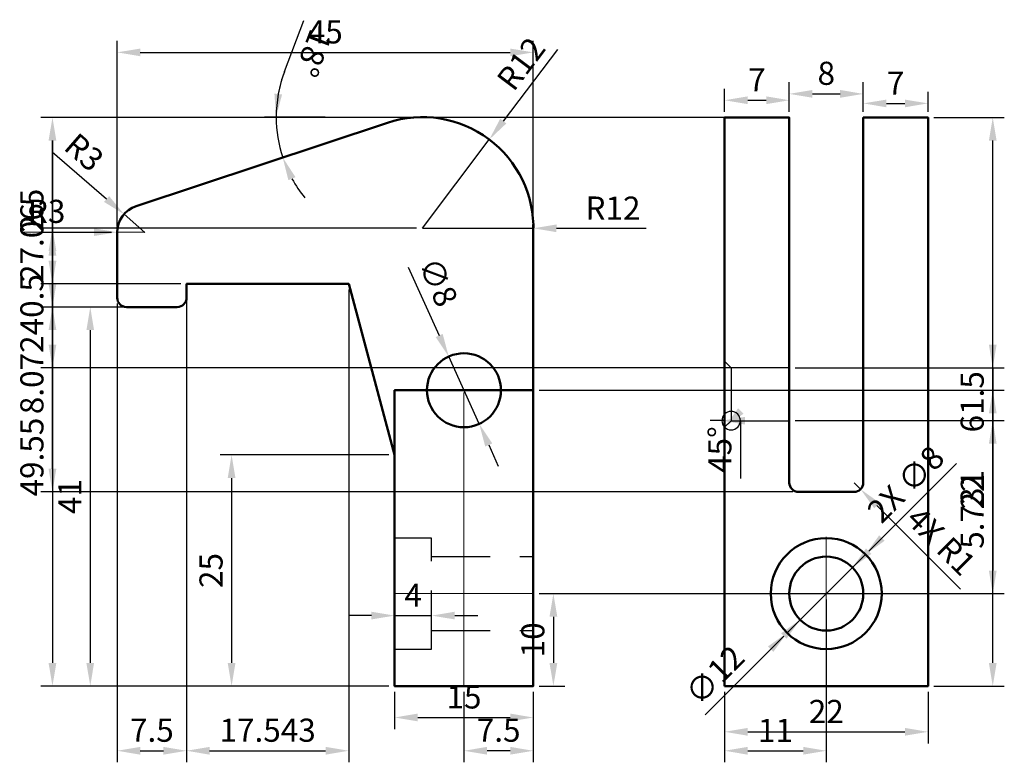
# Model space of a CAD drawing. Units: millimetres. Extents: x 28 to 135, y 8 to 88.
import ezdxf

# ---------------------------------------------------------------- set-up
doc = ezdxf.new("R2010")
doc.units = ezdxf.units.MM
doc.linetypes.add('CENTER', pattern=[50.8, 31.75, -6.35, 6.35, -6.35])
doc.linetypes.add('HIDDEN', pattern=[9.525, 6.35, -3.175])
for name, color, linetype, lineweight in [('M-CNTR', 4, 'CENTER', 18), ('M-CONS', 8, 'Continuous', 13), ('M-DIMS', 2, 'Continuous', 25), ('M-HIDN', 3, 'HIDDEN', 25), ('M-OUTL', 7, 'Continuous', 50)]:
    doc.layers.add(name, color=color, linetype=linetype, lineweight=lineweight)
doc.styles.get("Standard").update_dxf_attribs({"font": 'arial.ttf'})
doc.dimstyles.new('ISO-25', dxfattribs={"dimtxt": 2.5, "dimasz": 2.5, "dimexe": 1.25, "dimexo": 0.625, "dimtad": 1, "dimdec": 0, "dimtxsty": 'Standard', "dimcen": 2.5, "dimadec": 0, "dimazin": 0, "dimtfac": 1, "dimtdec": 0, "dimtmove": 0, "dimatfit": 3, "dimfxl": 1, "dimarcsym": 0})

# ---------------------------------------------------------------- blocks, each defined once
blk = doc.blocks.new('*D1')
at = {"layer": 'Defpoints', "color": 0, "transparency": 16777216}
for p in [(79.03, 75.07), (71.8, 65.5)]:
    blk.add_point(p, dxfattribs=at)
at = {"layer": 'M-DIMS', "color": 0, "lineweight": -2, "transparency": 16777216}
for p, q in [((86.39, 84.8), (80.54, 77.07)), ((71.8, 65.5), (79.03, 75.07))]:
    blk.add_line(p, q, dxfattribs=at)
at = {"layer": 'M-DIMS', "color": 0, "transparency": 16777216}
blk.add_solid([(80.21, 77.32), (80.87, 76.81), (79.03, 75.07)], dxfattribs=at)
at = {"layer": 'M-DIMS', "color": 0, "transparency": 16777216, "insert": (82.72, 83.07), "char_height": 2.5, "attachment_point": 5, "rotation": 52.9202}
blk.add_mtext('R12', dxfattribs=at)
blk = doc.blocks.new('*D2')
at = {"layer": 'Defpoints', "color": 0, "transparency": 16777216}
for p in [(39.53, 66.99), (41.79, 65.02)]:
    blk.add_point(p, dxfattribs=at)
at = {"layer": 'M-DIMS', "color": 0, "lineweight": -2, "transparency": 16777216}
for p, q in [((31.77, 73.75), (37.64, 68.64)), ((41.79, 65.02), (39.53, 66.99))]:
    blk.add_line(p, q, dxfattribs=at)
at = {"layer": 'M-DIMS', "color": 0, "transparency": 16777216}
blk.add_solid([(37.92, 68.95), (37.37, 68.32), (39.53, 66.99)], dxfattribs=at)
at = {"layer": 'M-DIMS', "color": 0, "transparency": 16777216, "insert": (35.01, 73.45), "char_height": 2.5, "attachment_point": 5, "rotation": 318.9491}
blk.add_mtext('R3', dxfattribs=at)
blk = doc.blocks.new('*D3')
at = {"layer": 'Defpoints', "color": 0, "transparency": 16777216}
for p in [(61.9, 77.5), (68.02, 76.89), (71.8, 77.5), (56.3, 74.56), (40.84, 67.87)]:
    blk.add_point(p, dxfattribs=at)
at = {"layer": 'M-DIMS', "color": 0, "lineweight": -2, "transparency": 16777216}
for p, q in [((56.88, 82.42), (58.98, 87.95)), ((61.28, 77.5), (54.73, 77.5))]:
    blk.add_line(p, q, dxfattribs=at)
for start, end in [(159.2411, 180), (159.3264, 169.6632), (180, 198.3579), (208.6947, 219.0315)]:
    blk.add_arc((69.86, 77.5), 13.88, start, end, dxfattribs=at)
at = {"layer": 'M-DIMS', "color": 0, "transparency": 16777216}
for points in [[(56.62, 79.95), (55.79, 80.03), (55.98, 77.5)], [(57.3, 70.67), (58.07, 71), (56.69, 73.13)]]:
    blk.add_solid(points, dxfattribs=at)
at = {"layer": 'M-DIMS', "color": 0, "transparency": 16777216, "insert": (59.71, 84.51), "char_height": 2.5, "attachment_point": 5, "rotation": 249.2411}
blk.add_mtext('18°', dxfattribs=at)
blk = doc.blocks.new('*D4')
at = {"layer": 'Defpoints', "color": 0, "transparency": 16777216}
for p in [(39.79, 56.95), (35.88, 15.95), (68.79, 15.95)]:
    blk.add_point(p, dxfattribs=at)
at = {"layer": 'M-DIMS', "color": 0, "lineweight": -2, "transparency": 16777216}
for p, q in [((39.16, 56.95), (34.63, 56.95)), ((35.88, 54.45), (35.88, 18.45)), ((68.16, 15.95), (34.63, 15.95))]:
    blk.add_line(p, q, dxfattribs=at)
at = {"layer": 'M-DIMS', "color": 0, "transparency": 16777216}
for points in [[(35.46, 54.45), (36.29, 54.45), (35.88, 56.95)], [(35.46, 18.45), (36.29, 18.45), (35.88, 15.95)]]:
    blk.add_solid(points, dxfattribs=at)
at = {"layer": 'M-DIMS', "color": 0, "transparency": 16777216, "insert": (34, 36.45), "char_height": 2.5, "attachment_point": 5, "rotation": 90}
blk.add_mtext('41', dxfattribs=at)
blk = doc.blocks.new('*D5')
at = {"layer": 'Defpoints', "color": 0, "transparency": 16777216}
for p in [(68.79, 40.95), (51.16, 15.95), (68.79, 15.95)]:
    blk.add_point(p, dxfattribs=at)
at = {"layer": 'M-DIMS', "color": 0, "lineweight": -2, "transparency": 16777216}
for p, q in [((68.16, 40.95), (49.91, 40.95)), ((51.16, 38.45), (51.16, 18.45)), ((68.16, 15.95), (49.91, 15.95))]:
    blk.add_line(p, q, dxfattribs=at)
at = {"layer": 'M-DIMS', "color": 0, "transparency": 16777216}
for points in [[(50.74, 38.45), (51.58, 38.45), (51.16, 40.95)], [(50.74, 18.45), (51.58, 18.45), (51.16, 15.95)]]:
    blk.add_solid(points, dxfattribs=at)
at = {"layer": 'M-DIMS', "color": 0, "transparency": 16777216, "insert": (49.26, 28.45), "char_height": 2.5, "attachment_point": 5, "rotation": 90}
blk.add_mtext('25', dxfattribs=at)
blk = doc.blocks.new('*D6')
at = {"layer": 'Defpoints', "color": 0, "transparency": 16777216}
for p in [(72.79, 23.57), (68.79, 22.11), (72.79, 22.11)]:
    blk.add_point(p, dxfattribs=at)
at = {"layer": 'M-DIMS', "color": 0, "lineweight": -2, "transparency": 16777216}
for p, q in [((68.79, 22.74), (68.79, 24.82)), ((72.79, 22.74), (72.79, 24.82)), ((66.29, 23.57), (63.79, 23.57)), ((68.79, 23.57), (72.79, 23.57)), ((75.29, 23.57), (77.79, 23.57))]:
    blk.add_line(p, q, dxfattribs=at)
at = {"layer": 'M-DIMS', "color": 0, "transparency": 16777216}
for points in [[(66.29, 23.99), (66.29, 23.16), (68.79, 23.57)], [(75.29, 23.99), (75.29, 23.16), (72.79, 23.57)]]:
    blk.add_solid(points, dxfattribs=at)
at = {"layer": 'M-DIMS', "color": 0, "transparency": 16777216, "insert": (70.79, 25.45), "char_height": 2.5, "attachment_point": 5}
blk.add_mtext('4', dxfattribs=at)
blk = doc.blocks.new('*D7')
at = {"layer": 'Defpoints', "color": 0, "transparency": 16777216}
for p in [(83.79, 25.95), (83.79, 15.95), (85.96, 15.95)]:
    blk.add_point(p, dxfattribs=at)
at = {"layer": 'M-DIMS', "color": 0, "lineweight": -2, "transparency": 16777216}
for p, q in [((84.41, 25.95), (87.21, 25.95)), ((85.96, 23.45), (85.96, 18.45)), ((84.41, 15.95), (87.21, 15.95))]:
    blk.add_line(p, q, dxfattribs=at)
at = {"layer": 'M-DIMS', "color": 0, "transparency": 16777216}
for points in [[(85.54, 23.45), (86.38, 23.45), (85.96, 25.95)], [(85.54, 18.45), (86.38, 18.45), (85.96, 15.95)]]:
    blk.add_solid(points, dxfattribs=at)
at = {"layer": 'M-DIMS', "color": 0, "transparency": 16777216, "insert": (84.06, 20.95), "char_height": 2.5, "attachment_point": 5, "rotation": 90}
blk.add_mtext('10', dxfattribs=at)
blk = doc.blocks.new('*D8')
at = {"layer": 'Defpoints', "color": 0, "transparency": 16777216}
for p in [(68.79, 15.95), (83.79, 15.95), (83.79, 12.55)]:
    blk.add_point(p, dxfattribs=at)
at = {"layer": 'M-DIMS', "color": 0, "lineweight": -2, "transparency": 16777216}
for p, q in [((68.79, 15.33), (68.79, 11.3)), ((83.79, 15.33), (83.79, 11.3)), ((71.29, 12.55), (81.29, 12.55))]:
    blk.add_line(p, q, dxfattribs=at)
at = {"layer": 'M-DIMS', "color": 0, "transparency": 16777216}
for points in [[(71.29, 12.97), (71.29, 12.13), (68.79, 12.55)], [(81.29, 12.97), (81.29, 12.13), (83.79, 12.55)]]:
    blk.add_solid(points, dxfattribs=at)
at = {"layer": 'M-DIMS', "color": 0, "transparency": 16777216, "insert": (76.29, 14.45), "char_height": 2.5, "attachment_point": 5}
blk.add_mtext('15', dxfattribs=at)
blk = doc.blocks.new('*D9')
at = {"layer": 'Defpoints', "color": 0, "transparency": 16777216}
for p in [(74.64, 51.59), (77.94, 44.31)]:
    blk.add_point(p, dxfattribs=at)
at = {"layer": 'M-DIMS', "color": 0, "lineweight": -2, "transparency": 16777216}
for p, q in [((70.26, 61.26), (73.61, 53.87)), ((77.94, 44.31), (74.64, 51.59)), ((78.97, 42.03), (80, 39.75))]:
    blk.add_line(p, q, dxfattribs=at)
at = {"layer": 'M-DIMS', "color": 0, "transparency": 16777216}
for points in [[(73.99, 54.04), (73.23, 53.7), (74.64, 51.59)], [(79.35, 42.2), (78.59, 41.86), (77.94, 44.31)]]:
    blk.add_solid(points, dxfattribs=at)
at = {"layer": 'M-DIMS', "color": 0, "transparency": 16777216, "insert": (73.21, 59.52), "char_height": 2.5, "attachment_point": 5, "rotation": 294.3831}
blk.add_mtext('∅8', dxfattribs=at)
blk = doc.blocks.new('*D10')
at = {"layer": 'Defpoints', "color": 0, "transparency": 16777216}
for p in [(104.47, 15.95), (126.47, 15.95), (126.47, 11)]:
    blk.add_point(p, dxfattribs=at)
at = {"layer": 'M-DIMS', "color": 0, "lineweight": -2, "transparency": 16777216}
for p, q in [((104.47, 15.33), (104.47, 9.75)), ((126.47, 15.33), (126.47, 9.75)), ((106.97, 11), (123.97, 11))]:
    blk.add_line(p, q, dxfattribs=at)
at = {"layer": 'M-DIMS', "color": 0, "transparency": 16777216}
for points in [[(106.97, 11.42), (106.97, 10.58), (104.47, 11)], [(123.97, 11.42), (123.97, 10.58), (126.47, 11)]]:
    blk.add_solid(points, dxfattribs=at)
at = {"layer": 'M-DIMS', "color": 0, "transparency": 16777216, "insert": (115.47, 12.88), "char_height": 2.5, "attachment_point": 5}
blk.add_mtext('22', dxfattribs=at)
blk = doc.blocks.new('*D11')
at = {"layer": 'Defpoints', "color": 0, "transparency": 16777216}
for p in [(104.21, 44.4), (104.47, 43.95), (105.18, 44.66), (105.18, 44.66), (111.47, 44.66)]:
    blk.add_point(p, dxfattribs=at)
at = {"layer": 'M-DIMS', "color": 0, "lineweight": -2, "transparency": 16777216}
for p, q in [((104.55, 44.66), (102.93, 44.66)), ((106.18, 44.66), (106.18, 38.4))]:
    blk.add_line(p, q, dxfattribs=at)
for start, end in [(360, 180), (45, 225), (180, 360), (180, 225)]:
    blk.add_arc((105.18, 44.66), 1, start, end, dxfattribs=at)
at = {"layer": 'M-DIMS', "color": 0, "transparency": 16777216}
for points in [[(106.53, 45.42), (105.94, 46.01), (104.47, 43.95)], [(106.68, 44.24), (106.68, 45.07), (104.18, 44.66)]]:
    blk.add_solid(points, dxfattribs=at)
at = {"layer": 'M-DIMS', "color": 0, "transparency": 16777216, "insert": (104.28, 41.53), "char_height": 2.5, "attachment_point": 5, "rotation": 90}
blk.add_mtext('45°', dxfattribs=at)
blk = doc.blocks.new('*D12')
at = {"layer": 'Defpoints', "color": 0, "transparency": 16777216}
for p in [(111.47, 79.32), (104.47, 77.45), (111.47, 77.45)]:
    blk.add_point(p, dxfattribs=at)
at = {"layer": 'M-DIMS', "color": 0, "lineweight": -2, "transparency": 16777216}
for p, q in [((104.47, 78.08), (104.47, 80.57)), ((111.47, 78.08), (111.47, 80.57)), ((106.97, 79.32), (108.97, 79.32))]:
    blk.add_line(p, q, dxfattribs=at)
at = {"layer": 'M-DIMS', "color": 0, "transparency": 16777216}
for points in [[(106.97, 79.74), (106.97, 78.9), (104.47, 79.32)], [(108.97, 79.74), (108.97, 78.9), (111.47, 79.32)]]:
    blk.add_solid(points, dxfattribs=at)
at = {"layer": 'M-DIMS', "color": 0, "transparency": 16777216, "insert": (107.97, 81.2), "char_height": 2.5, "attachment_point": 5}
blk.add_mtext('7', dxfattribs=at)
blk = doc.blocks.new('*D13')
at = {"layer": 'Defpoints', "color": 0, "transparency": 16777216}
for p in [(119.47, 80.01), (111.47, 77.45), (119.47, 77.45)]:
    blk.add_point(p, dxfattribs=at)
at = {"layer": 'M-DIMS', "color": 0, "lineweight": -2, "transparency": 16777216}
for p, q in [((111.47, 78.08), (111.47, 81.26)), ((119.47, 78.08), (119.47, 81.26)), ((113.97, 80.01), (116.97, 80.01))]:
    blk.add_line(p, q, dxfattribs=at)
at = {"layer": 'M-DIMS', "color": 0, "transparency": 16777216}
for points in [[(113.97, 80.43), (113.97, 79.59), (111.47, 80.01)], [(116.97, 80.43), (116.97, 79.59), (119.47, 80.01)]]:
    blk.add_solid(points, dxfattribs=at)
at = {"layer": 'M-DIMS', "color": 0, "transparency": 16777216, "insert": (115.47, 81.91), "char_height": 2.5, "attachment_point": 5}
blk.add_mtext('8', dxfattribs=at)
blk = doc.blocks.new('*D14')
at = {"layer": 'Defpoints', "color": 0, "transparency": 16777216}
for p in [(126.47, 78.98), (119.47, 77.45), (126.47, 77.45)]:
    blk.add_point(p, dxfattribs=at)
at = {"layer": 'M-DIMS', "color": 0, "lineweight": -2, "transparency": 16777216}
for p, q in [((119.47, 78.08), (119.47, 80.23)), ((126.47, 78.08), (126.47, 80.23)), ((121.97, 78.98), (123.97, 78.98))]:
    blk.add_line(p, q, dxfattribs=at)
at = {"layer": 'M-DIMS', "color": 0, "transparency": 16777216}
for points in [[(121.97, 79.39), (121.97, 78.56), (119.47, 78.98)], [(123.97, 79.39), (123.97, 78.56), (126.47, 78.98)]]:
    blk.add_solid(points, dxfattribs=at)
at = {"layer": 'M-DIMS', "color": 0, "transparency": 16777216, "insert": (122.97, 80.85), "char_height": 2.5, "attachment_point": 5}
blk.add_mtext('7', dxfattribs=at)
blk = doc.blocks.new('*D15')
at = {"layer": 'Defpoints', "color": 0, "transparency": 16777216}
for p in [(83.79, 84.5), (38.79, 65.02), (83.79, 65.11)]:
    blk.add_point(p, dxfattribs=at)
at = {"layer": 'M-DIMS', "color": 0, "lineweight": -2, "transparency": 16777216}
for p, q in [((38.79, 65.65), (38.79, 85.75)), ((83.79, 65.73), (83.79, 85.75)), ((41.29, 84.5), (81.29, 84.5))]:
    blk.add_line(p, q, dxfattribs=at)
at = {"layer": 'M-DIMS', "color": 0, "transparency": 16777216}
for points in [[(41.29, 84.91), (41.29, 84.08), (38.79, 84.5)], [(81.29, 84.91), (81.29, 84.08), (83.79, 84.5)]]:
    blk.add_solid(points, dxfattribs=at)
at = {"layer": 'M-DIMS', "color": 0, "transparency": 16777216, "insert": (61.29, 86.39), "char_height": 2.5, "attachment_point": 5}
blk.add_mtext('45', dxfattribs=at)
blk = doc.blocks.new('*D16')
at = {"layer": 'Defpoints', "color": 0, "transparency": 16777216}
for p in [(126.47, 77.45), (133.47, 77.45), (126.47, 15.95)]:
    blk.add_point(p, dxfattribs=at)
at = {"layer": 'M-DIMS', "color": 0, "lineweight": -2, "transparency": 16777216}
for p, q in [((127.1, 77.45), (134.72, 77.45)), ((133.47, 18.45), (133.47, 74.95)), ((127.1, 15.95), (134.72, 15.95))]:
    blk.add_line(p, q, dxfattribs=at)
at = {"layer": 'M-DIMS', "color": 0, "transparency": 16777216}
for points in [[(133.05, 74.95), (133.89, 74.95), (133.47, 77.45)], [(133.05, 18.45), (133.89, 18.45), (133.47, 15.95)]]:
    blk.add_solid(points, dxfattribs=at)
at = {"layer": 'M-DIMS', "color": 0, "transparency": 16777216, "insert": (131.57, 46.7), "char_height": 2.5, "attachment_point": 5, "rotation": 90}
blk.add_mtext('61.5', dxfattribs=at)
blk = doc.blocks.new('*D17')
at = {"layer": 'Defpoints', "color": 0, "transparency": 16777216}
for p in [(71.8, 65.5), (31.79, 15.95), (68.79, 15.95)]:
    blk.add_point(p, dxfattribs=at)
at = {"layer": 'M-DIMS', "color": 0, "lineweight": -2, "transparency": 16777216}
for p, q in [((71.17, 65.5), (30.54, 65.5)), ((31.79, 63), (31.79, 18.45)), ((68.16, 15.95), (30.54, 15.95))]:
    blk.add_line(p, q, dxfattribs=at)
at = {"layer": 'M-DIMS', "color": 0, "transparency": 16777216}
for points in [[(31.37, 63), (32.21, 63), (31.79, 65.5)], [(31.37, 18.45), (32.21, 18.45), (31.79, 15.95)]]:
    blk.add_solid(points, dxfattribs=at)
at = {"layer": 'M-DIMS', "color": 0, "transparency": 16777216, "insert": (29.89, 40.72), "char_height": 2.5, "attachment_point": 5, "rotation": 90}
blk.add_mtext('49.55', dxfattribs=at)
blk = doc.blocks.new('*D18')
at = {"layer": 'Defpoints', "color": 0, "transparency": 16777216}
for p in [(83.79, 47.95), (83.79, 25.95), (133.47, 25.95)]:
    blk.add_point(p, dxfattribs=at)
at = {"layer": 'M-DIMS', "color": 0, "lineweight": -2, "transparency": 16777216}
for p, q in [((84.41, 47.95), (134.72, 47.95)), ((133.47, 45.45), (133.47, 28.45)), ((84.41, 25.95), (134.72, 25.95))]:
    blk.add_line(p, q, dxfattribs=at)
at = {"layer": 'M-DIMS', "color": 0, "transparency": 16777216}
for points in [[(133.05, 45.45), (133.89, 45.45), (133.47, 47.95)], [(133.05, 28.45), (133.89, 28.45), (133.47, 25.95)]]:
    blk.add_solid(points, dxfattribs=at)
at = {"layer": 'M-DIMS', "color": 0, "transparency": 16777216, "insert": (131.59, 36.95), "char_height": 2.5, "attachment_point": 5, "rotation": 90}
blk.add_mtext('22', dxfattribs=at)
blk = doc.blocks.new('*D19')
at = {"layer": 'Defpoints', "color": 0, "transparency": 16777216}
for p in [(31.79, 77.45), (111.47, 77.45), (112.47, 36.95)]:
    blk.add_point(p, dxfattribs=at)
at = {"layer": 'M-DIMS', "color": 0, "lineweight": -2, "transparency": 16777216}
for p, q in [((110.85, 77.45), (30.54, 77.45)), ((31.79, 39.45), (31.79, 74.95)), ((111.85, 36.95), (30.54, 36.95))]:
    blk.add_line(p, q, dxfattribs=at)
at = {"layer": 'M-DIMS', "color": 0, "transparency": 16777216}
for points in [[(31.37, 74.95), (32.21, 74.95), (31.79, 77.45)], [(31.37, 39.45), (32.21, 39.45), (31.79, 36.95)]]:
    blk.add_solid(points, dxfattribs=at)
at = {"layer": 'M-DIMS', "color": 0, "transparency": 16777216, "insert": (29.89, 57.2), "char_height": 2.5, "attachment_point": 5, "rotation": 90}
blk.add_mtext('40.5', dxfattribs=at)
blk = doc.blocks.new('*D20')
at = {"layer": 'Defpoints', "color": 0, "transparency": 16777216}
for p in [(76.29, 15.95), (83.79, 15.95), (76.29, 8.95)]:
    blk.add_point(p, dxfattribs=at)
at = {"layer": 'M-DIMS', "color": 0, "lineweight": -2, "transparency": 16777216}
for p, q in [((76.29, 15.33), (76.29, 7.7)), ((83.79, 15.33), (83.79, 7.7)), ((81.29, 8.95), (78.79, 8.95))]:
    blk.add_line(p, q, dxfattribs=at)
at = {"layer": 'M-DIMS', "color": 0, "transparency": 16777216}
for points in [[(78.79, 9.37), (78.79, 8.53), (76.29, 8.95)], [(81.29, 9.37), (81.29, 8.53), (83.79, 8.95)]]:
    blk.add_solid(points, dxfattribs=at)
at = {"layer": 'M-DIMS', "color": 0, "transparency": 16777216, "insert": (80.04, 10.85), "char_height": 2.5, "attachment_point": 5}
blk.add_mtext('7.5', dxfattribs=at)
blk = doc.blocks.new('*D21')
at = {"layer": 'Defpoints', "color": 0, "transparency": 16777216}
for p in [(115.47, 25.95), (104.47, 15.95), (115.47, 8.95)]:
    blk.add_point(p, dxfattribs=at)
at = {"layer": 'M-DIMS', "color": 0, "lineweight": -2, "transparency": 16777216}
for p, q in [((115.47, 25.33), (115.47, 7.7)), ((104.47, 15.33), (104.47, 7.7)), ((106.97, 8.95), (112.97, 8.95))]:
    blk.add_line(p, q, dxfattribs=at)
at = {"layer": 'M-DIMS', "color": 0, "transparency": 16777216}
for points in [[(106.97, 9.37), (106.97, 8.53), (104.47, 8.95)], [(112.97, 9.37), (112.97, 8.53), (115.47, 8.95)]]:
    blk.add_solid(points, dxfattribs=at)
at = {"layer": 'M-DIMS', "color": 0, "transparency": 16777216, "insert": (109.97, 10.83), "char_height": 2.5, "attachment_point": 5}
blk.add_mtext('11', dxfattribs=at)
blk = doc.blocks.new('*D22')
at = {"layer": 'Defpoints', "color": 0, "transparency": 16777216}
for p in [(46.29, 59.45), (38.79, 57.95), (46.29, 8.95)]:
    blk.add_point(p, dxfattribs=at)
at = {"layer": 'M-DIMS', "color": 0, "lineweight": -2, "transparency": 16777216}
for p, q in [((46.29, 58.83), (46.29, 7.7)), ((38.79, 57.33), (38.79, 7.7)), ((41.29, 8.95), (43.79, 8.95))]:
    blk.add_line(p, q, dxfattribs=at)
at = {"layer": 'M-DIMS', "color": 0, "transparency": 16777216}
for points in [[(41.29, 9.37), (41.29, 8.53), (38.79, 8.95)], [(43.79, 9.37), (43.79, 8.53), (46.29, 8.95)]]:
    blk.add_solid(points, dxfattribs=at)
at = {"layer": 'M-DIMS', "color": 0, "transparency": 16777216, "insert": (42.54, 10.85), "char_height": 2.5, "attachment_point": 5}
blk.add_mtext('7.5', dxfattribs=at)
blk = doc.blocks.new('*D23')
at = {"layer": 'Defpoints', "color": 0, "transparency": 16777216}
for p in [(31.79, 59.45), (46.29, 59.45), (45.29, 56.95)]:
    blk.add_point(p, dxfattribs=at)
at = {"layer": 'M-DIMS', "color": 0, "lineweight": -2, "transparency": 16777216}
for p, q in [((31.79, 61.95), (31.79, 70.31)), ((45.66, 59.45), (30.54, 59.45)), ((31.79, 56.95), (31.79, 59.45)), ((44.66, 56.95), (30.54, 56.95)), ((31.79, 54.45), (31.79, 51.95))]:
    blk.add_line(p, q, dxfattribs=at)
at = {"layer": 'M-DIMS', "color": 0, "transparency": 16777216}
for points in [[(31.37, 61.95), (32.21, 61.95), (31.79, 59.45)], [(31.37, 54.45), (32.21, 54.45), (31.79, 56.95)]]:
    blk.add_solid(points, dxfattribs=at)
at = {"layer": 'M-DIMS', "color": 0, "transparency": 16777216, "insert": (29.89, 67.38), "char_height": 2.5, "attachment_point": 5, "rotation": 90}
blk.add_mtext('2.5', dxfattribs=at)
blk = doc.blocks.new('*D24')
at = {"layer": 'Defpoints', "color": 0, "transparency": 16777216}
for p in [(46.29, 59.45), (63.83, 59.45), (63.83, 8.95)]:
    blk.add_point(p, dxfattribs=at)
at = {"layer": 'M-DIMS', "color": 0, "lineweight": -2, "transparency": 16777216}
for p, q in [((46.29, 58.83), (46.29, 7.7)), ((63.83, 58.83), (63.83, 7.7)), ((48.79, 8.95), (61.33, 8.95))]:
    blk.add_line(p, q, dxfattribs=at)
at = {"layer": 'M-DIMS', "color": 0, "transparency": 16777216}
for points in [[(48.79, 9.37), (48.79, 8.53), (46.29, 8.95)], [(61.33, 9.37), (61.33, 8.53), (63.83, 8.95)]]:
    blk.add_solid(points, dxfattribs=at)
at = {"layer": 'M-DIMS', "color": 0, "transparency": 16777216, "insert": (55.06, 10.85), "char_height": 2.5, "attachment_point": 5}
blk.add_mtext('17.543', dxfattribs=at)
blk = doc.blocks.new('*D25')
at = {"layer": 'Defpoints', "color": 0, "transparency": 16777216}
for p in [(38.79, 65.02), (31.79, 56.95), (39.79, 56.95)]:
    blk.add_point(p, dxfattribs=at)
at = {"layer": 'M-DIMS', "color": 0, "lineweight": -2, "transparency": 16777216}
for p, q in [((38.16, 65.02), (30.54, 65.02)), ((31.79, 62.52), (31.79, 59.45)), ((39.16, 56.95), (30.54, 56.95)), ((31.79, 56.95), (31.79, 44.79))]:
    blk.add_line(p, q, dxfattribs=at)
at = {"layer": 'M-DIMS', "color": 0, "transparency": 16777216}
for points in [[(31.37, 62.52), (32.21, 62.52), (31.79, 65.02)], [(31.37, 59.45), (32.21, 59.45), (31.79, 56.95)]]:
    blk.add_solid(points, dxfattribs=at)
at = {"layer": 'M-DIMS', "color": 0, "transparency": 16777216, "insert": (29.89, 49.62), "char_height": 2.5, "attachment_point": 5, "rotation": 90}
blk.add_mtext('8.072', dxfattribs=at)
blk = doc.blocks.new('*D26')
at = {"layer": 'Defpoints', "color": 0, "transparency": 16777216}
for p in [(111.47, 77.45), (31.79, 50.39), (111.47, 50.39)]:
    blk.add_point(p, dxfattribs=at)
at = {"layer": 'M-DIMS', "color": 0, "lineweight": -2, "transparency": 16777216}
for p, q in [((110.85, 77.45), (30.54, 77.45)), ((31.79, 74.95), (31.79, 52.89)), ((110.85, 50.39), (30.54, 50.39))]:
    blk.add_line(p, q, dxfattribs=at)
at = {"layer": 'M-DIMS', "color": 0, "transparency": 16777216}
for points in [[(31.37, 74.95), (32.21, 74.95), (31.79, 77.45)], [(31.37, 52.89), (32.21, 52.89), (31.79, 50.39)]]:
    blk.add_solid(points, dxfattribs=at)
at = {"layer": 'M-DIMS', "color": 0, "transparency": 16777216, "insert": (29.89, 63.92), "char_height": 2.5, "attachment_point": 5, "rotation": 90}
blk.add_mtext('27.06', dxfattribs=at)
blk = doc.blocks.new('*D27')
at = {"layer": 'Defpoints', "color": 0, "transparency": 16777216}
for p in [(111.47, 50.39), (111.47, 44.66), (133.47, 44.66)]:
    blk.add_point(p, dxfattribs=at)
at = {"layer": 'M-DIMS', "color": 0, "lineweight": -2, "transparency": 16777216}
for p, q in [((133.47, 52.89), (133.47, 55.39)), ((112.1, 50.39), (134.72, 50.39)), ((133.47, 50.39), (133.47, 44.66)), ((112.1, 44.66), (134.72, 44.66)), ((133.47, 42.16), (133.47, 30.45))]:
    blk.add_line(p, q, dxfattribs=at)
at = {"layer": 'M-DIMS', "color": 0, "transparency": 16777216}
for points in [[(133.05, 52.89), (133.89, 52.89), (133.47, 50.39)], [(133.05, 42.16), (133.89, 42.16), (133.47, 44.66)]]:
    blk.add_solid(points, dxfattribs=at)
at = {"layer": 'M-DIMS', "color": 0, "transparency": 16777216, "insert": (131.57, 35.06), "char_height": 2.5, "attachment_point": 5, "rotation": 90}
blk.add_mtext('5.731', dxfattribs=at)
blk = doc.blocks.new('*D28')
at = {"layer": 'Defpoints', "color": 0, "transparency": 16777216}
for p in [(71.8, 65.5), (83.8, 65.47)]:
    blk.add_point(p, dxfattribs=at)
at = {"layer": 'M-DIMS', "color": 0, "lineweight": -2, "transparency": 16777216}
for p, q in [((71.8, 65.5), (83.8, 65.47)), ((95.99, 65.44), (86.3, 65.46))]:
    blk.add_line(p, q, dxfattribs=at)
at = {"layer": 'M-DIMS', "color": 0, "transparency": 16777216}
blk.add_solid([(86.3, 65.88), (86.29, 65.05), (83.8, 65.47)], dxfattribs=at)
at = {"layer": 'M-DIMS', "color": 0, "transparency": 16777216, "insert": (92.4, 67.33), "char_height": 2.5, "attachment_point": 5, "rotation": 359.8656}
blk.add_mtext('R12', dxfattribs=at)
blk = doc.blocks.new('*D29')
at = {"layer": 'Defpoints', "color": 0, "transparency": 16777216}
for p in [(38.79, 65.04), (41.79, 65.02)]:
    blk.add_point(p, dxfattribs=at)
at = {"layer": 'M-DIMS', "color": 0, "lineweight": -2, "transparency": 16777216}
for p, q in [((28.51, 65.1), (36.29, 65.05)), ((41.79, 65.02), (38.79, 65.04))]:
    blk.add_line(p, q, dxfattribs=at)
at = {"layer": 'M-DIMS', "color": 0, "transparency": 16777216}
blk.add_solid([(36.29, 65.47), (36.29, 64.64), (38.79, 65.04)], dxfattribs=at)
at = {"layer": 'M-DIMS', "color": 0, "transparency": 16777216, "insert": (31.16, 66.98), "char_height": 2.5, "attachment_point": 5, "rotation": 359.6837}
blk.add_mtext('R3', dxfattribs=at)
blk = doc.blocks.new('*D30')
at = {"layer": 'Defpoints', "color": 0, "transparency": 16777216}
for p in [(118.47, 37.95), (119.18, 37.24)]:
    blk.add_point(p, dxfattribs=at)
at = {"layer": 'M-DIMS', "color": 0, "lineweight": -2, "transparency": 16777216}
for p, q in [((118.47, 37.95), (119.18, 37.24)), ((129.97, 26.44), (120.94, 35.48))]:
    blk.add_line(p, q, dxfattribs=at)
at = {"layer": 'M-DIMS', "color": 0, "transparency": 16777216}
blk.add_solid([(121.24, 35.77), (120.65, 35.18), (119.18, 37.24)], dxfattribs=at)
at = {"layer": 'M-DIMS', "color": 0, "transparency": 16777216, "insert": (127.67, 31.41), "char_height": 2.5, "attachment_point": 5, "rotation": 314.995}
blk.add_mtext('4X R1', dxfattribs=at)
blk = doc.blocks.new('*D31')
at = {"layer": 'Defpoints', "color": 0, "transparency": 16777216}
for p in [(118.3, 28.78), (112.64, 23.12)]:
    blk.add_point(p, dxfattribs=at)
at = {"layer": 'M-DIMS', "color": 0, "lineweight": -2, "transparency": 16777216}
for p, q in [((129.54, 40.02), (120.07, 30.55)), ((112.64, 23.12), (118.3, 28.78)), ((110.87, 21.35), (109.11, 19.59))]:
    blk.add_line(p, q, dxfattribs=at)
at = {"layer": 'M-DIMS', "color": 0, "transparency": 16777216}
for points in [[(119.77, 30.84), (120.36, 30.25), (118.3, 28.78)], [(110.58, 21.65), (111.17, 21.06), (112.64, 23.12)]]:
    blk.add_solid(points, dxfattribs=at)
at = {"layer": 'M-DIMS', "color": 0, "transparency": 16777216, "insert": (124.29, 37.56), "char_height": 2.5, "attachment_point": 5, "rotation": 45.0004}
blk.add_mtext('2X ∅8', dxfattribs=at)
blk = doc.blocks.new('*D32')
at = {"layer": 'Defpoints', "color": 0, "transparency": 16777216}
for p in [(119.71, 30.19), (111.23, 21.71)]:
    blk.add_point(p, dxfattribs=at)
at = {"layer": 'M-DIMS', "color": 0, "lineweight": -2, "transparency": 16777216}
for p, q in [((121.48, 31.96), (123.25, 33.73)), ((119.71, 30.19), (111.23, 21.71)), ((102.37, 12.85), (109.46, 19.94))]:
    blk.add_line(p, q, dxfattribs=at)
at = {"layer": 'M-DIMS', "color": 0, "transparency": 16777216}
for points in [[(121.19, 32.26), (121.78, 31.67), (119.71, 30.19)], [(109.17, 20.24), (109.75, 19.65), (111.23, 21.71)]]:
    blk.add_solid(points, dxfattribs=at)
at = {"layer": 'M-DIMS', "color": 0, "transparency": 16777216, "insert": (103.64, 16.91), "char_height": 2.5, "attachment_point": 5, "rotation": 44.9997}
blk.add_mtext('∅12', dxfattribs=at)

msp = doc.modelspace()

# ---------------------------------------------------------------- linework, layer by layer
at = {"layer": 'M-CNTR'}
for p, q in [((76.2893, 15.951), (76.2893, 47.951)), ((115.4701, 15.951), (115.4701, 32.0972)), ((68.7893, 25.951), (83.7893, 25.951)), ((108.1671, 25.951), (121.4149, 25.951))]:
    msp.add_line(p, q, dxfattribs=at)
at = {"layer": 'M-CONS'}
msp.add_line((71.7956, 77.4981), (61.9014, 77.4981), dxfattribs=at)
at = {"layer": 'M-HIDN'}
for p, q in [((104.4701, 51.0967), (105.1772, 50.3896)), ((104.4701, 43.951), (105.1772, 44.6581)), ((72.7893, 29.951), (83.7893, 29.951)), ((72.7893, 21.951), (83.7893, 21.951))]:
    msp.add_line(p, q, dxfattribs=at)
for points in [[(111.4701, 50.3896), (105.1772, 50.3896), (105.1772, 44.6581), (111.4701, 44.6581)], [(68.7893, 19.951), (72.7893, 19.951), (72.7893, 31.951), (68.7893, 31.951)]]:
    msp.add_lwpolyline(points, dxfattribs=at)
at = {"layer": 'M-OUTL'}
msp.add_lwpolyline([(83.7893, 47.951), (83.7893, 15.951), (68.7893, 15.951), (68.7893, 40.951), (63.8322, 59.451), (46.2893, 59.451), (46.2893, 57.951, -0.41421356), (45.2893, 56.951), (39.7893, 56.951, -0.41421356), (38.7893, 57.951), (38.7893, 65.0234, -0.32319407), (40.8444, 67.8708), (68.0161, 76.8874, -0.52174073), (83.7893, 65.11)], format="xyb", dxfattribs=at)
msp.add_lwpolyline([(104.4701, 15.951), (126.4701, 15.951), (126.4701, 77.451), (119.4701, 77.451), (119.4701, 37.951, -0.41421356), (118.4701, 36.951), (112.4701, 36.951, -0.41421356), (111.4701, 37.951), (111.4701, 77.451), (104.4701, 77.451)], format="xyb", close=True, dxfattribs=at)
msp.add_lwpolyline([(68.7893, 40.951), (68.7893, 47.951), (83.7893, 47.951), (83.7893, 65.8863)], dxfattribs=at)
for centre, radius in [((76.2893, 47.951), 4), ((115.4701, 25.951), 6), ((115.4701, 25.951), 4)]:
    msp.add_circle(centre, radius, dxfattribs=at)

# ---------------------------------------------------------------- dimensions: what is measured, and where the dimension line sits
at = {"layer": 'M-DIMS'}
for base, p1, p2, override, picture, middle in [((83.7893, 84.4981), (38.7893, 65.0234), (83.7893, 65.11), {"dimdec": 0, "dimlfac": 1, "dimrnd": 0, "dimzin": 0, "dimdsep": 46, "dimlunit": 2}, '*D15', (61.2893, 86.3944)), ((119.4701, 80.0113), (111.4701, 77.451), (119.4701, 77.451), {"dimclrd": 0, "dimclre": 0, "dimclrt": 0}, '*D13', (115.4701, 81.9127)), ((111.4701, 79.3213), (104.4701, 77.451), (111.4701, 77.451), {"dimclrd": 0, "dimclre": 0, "dimclrt": 0}, '*D12', (107.9701, 81.1963)), ((126.4701, 78.9762), (119.4701, 77.451), (126.4701, 77.451), {"dimclrd": 0, "dimclre": 0, "dimclrt": 0}, '*D14', (122.9701, 80.8512)), ((46.2893, 8.951), (38.7893, 57.951), (46.2893, 59.451), {"dimdec": 1, "dimlfac": 1, "dimrnd": 0, "dimzin": 0, "dimdsep": 46, "dimlunit": 2}, '*D22', (42.5393, 10.8474)), ((63.8322, 8.951), (46.2893, 59.451), (63.8322, 59.451), {"dimdec": 3, "dimlfac": 1, "dimrnd": 0, "dimzin": 0, "dimdsep": 46, "dimlunit": 2}, '*D24', (55.0607, 10.8533)), ((72.7893, 23.5742), (68.7893, 22.1108), (72.7893, 22.1108), {"dimclrd": 0, "dimclre": 0, "dimclrt": 0}, '*D6', (70.7893, 25.4492)), ((115.4701, 8.951), (104.4701, 15.951), (115.4701, 25.951), {"dimdec": 0, "dimlfac": 1, "dimrnd": 0, "dimzin": 0, "dimdsep": 46, "dimlunit": 2}, '*D21', (109.9701, 10.8312)), ((83.7893, 12.5498), (68.7893, 15.951), (83.7893, 15.951), {"dimclrd": 0, "dimclre": 0, "dimclrt": 0}, '*D8', (76.2893, 14.4512)), ((76.2893, 8.951), (83.7893, 15.951), (76.2893, 15.951), {"dimdec": 1, "dimlfac": 1, "dimrnd": 0, "dimzin": 0, "dimdsep": 46, "dimlunit": 2}, '*D20', (80.0393, 10.8474)), ((126.4701, 10.9987), (104.4701, 15.951), (126.4701, 15.951), {"dimclrd": 0, "dimclre": 0, "dimclrt": 0}, '*D10', (115.4701, 12.8789))]:
    dim = msp.add_linear_dim(base=base, p1=p1, p2=p2, dimstyle='ISO-25', override=override, dxfattribs=at)
    dim.commit()
    dim.dimension.update_dxf_attribs({"geometry": picture, "text_midpoint": middle})
for base, line1, line2, picture, middle in [((56.2958, 74.5566), ((40.8444, 67.8708), (68.0161, 76.8874)), ((71.7956, 77.4981), (61.9014, 77.4981)), '*D3', (59.7083, 84.5098)), ((104.2113, 44.3993), ((105.1772, 44.6581), (111.4701, 44.6581)), ((104.4701, 43.951), (105.1772, 44.6581)), '*D11', (104.2809, 41.5306))]:
    dim = msp.add_angular_dim_2l(base=base, line1=line1, line2=line2, dimstyle='ISO-25', override={"dimclrd": 0, "dimclre": 0, "dimclrt": 0}, dxfattribs=at)
    dim.commit()
    dim.dimension.update_dxf_attribs({"geometry": picture, "text_midpoint": middle})
for center, mpoint, override, picture, middle in [((71.7956, 65.4981), (79.0307, 75.0717), {"dimclrd": 0, "dimclre": 0, "dimclrt": 0}, '*D1', (82.7153, 83.0656)), ((41.7893, 65.0234), (39.5269, 66.9936), {"dimclrd": 0, "dimclre": 0, "dimclrt": 0}, '*D2', (35.0141, 73.446)), ((41.7893, 65.0234), (38.7893, 65.04), {"dimdec": 0, "dimlfac": 1, "dimrnd": 0, "dimzin": 0, "dimdsep": 46, "dimlunit": 2}, '*D29', (31.1593, 66.9844)), ((71.7956, 65.4981), (83.7955, 65.47), {"dimdec": 0, "dimlfac": 1, "dimrnd": 0, "dimzin": 0, "dimdsep": 46, "dimlunit": 2}, '*D28', (92.399, 67.3299))]:
    dim = msp.add_radius_dim(center=center, mpoint=mpoint, dimstyle='ISO-25', override=override, dxfattribs=at)
    dim.commit()
    dim.dimension.update_dxf_attribs({"geometry": picture, "text_midpoint": middle})
for base, p1, p2, override, picture, middle in [((31.7893, 77.451), (112.4701, 36.951), (111.4701, 77.451), {"dimdec": 1, "dimlfac": 1, "dimrnd": 0, "dimzin": 0, "dimdsep": 46, "dimlunit": 2}, '*D19', (29.8878, 57.201)), ((31.7893, 50.3896), (111.4701, 77.451), (111.4701, 50.3896), {"dimdec": 2, "dimlfac": 1, "dimrnd": 0, "dimzin": 0, "dimdsep": 46, "dimlunit": 2}, '*D26', (29.8878, 63.9203)), ((133.4701, 77.451), (126.4701, 15.951), (126.4701, 77.451), {"dimdec": 1, "dimlfac": 1, "dimrnd": 0, "dimzin": 0, "dimdsep": 46, "dimlunit": 2}, '*D16', (131.5686, 46.701)), ((31.7893, 59.451), (45.2893, 56.951), (46.2893, 59.451), {"dimdec": 1, "dimlfac": 1, "dimrnd": 0, "dimzin": 0, "dimdsep": 46, "dimlunit": 2}, '*D23', (29.8878, 67.3825)), ((31.7893, 15.951), (71.7956, 65.4981), (68.7893, 15.951), {"dimdec": 2, "dimlfac": 1, "dimrnd": 0, "dimzin": 0, "dimdsep": 46, "dimlunit": 2}, '*D17', (29.8878, 40.7246)), ((31.7893, 56.951), (38.7893, 65.0234), (39.7893, 56.951), {"dimdec": 3, "dimlfac": 1, "dimrnd": 0, "dimzin": 0, "dimdsep": 46, "dimlunit": 2}, '*D25', (29.8878, 49.619)), ((35.8768, 15.951), (39.7893, 56.951), (68.7893, 15.951), {"dimclrd": 0, "dimclre": 0, "dimclrt": 0}, '*D4', (33.9967, 36.451)), ((133.47008, 44.65815), (111.47008, 50.38958), (111.47008, 44.65815), {"dimdec": 3, "dimlfac": 1, "dimrnd": 0, "dimzin": 0, "dimdsep": 46, "dimlunit": 2}, '*D27', (131.5678, 35.05634)), ((133.4701, 25.951), (83.7893, 47.951), (83.7893, 25.951), {"dimdec": 0, "dimlfac": 1, "dimrnd": 0, "dimzin": 0, "dimdsep": 46, "dimlunit": 2}, '*D18', (131.59, 36.951)), ((51.1601, 15.951), (68.7893, 40.951), (68.7893, 15.951), {"dimclrd": 0, "dimclre": 0, "dimclrt": 0}, '*D5', (49.2587, 28.451)), ((85.9592, 15.951), (83.7893, 25.951), (83.7893, 15.951), {"dimclrd": 0, "dimclre": 0, "dimclrt": 0}, '*D7', (84.0577, 20.951))]:
    dim = msp.add_linear_dim(base=base, p1=p1, p2=p2, angle=90, dimstyle='ISO-25', override=override, dxfattribs=at)
    dim.commit()
    dim.dimension.update_dxf_attribs({"geometry": picture, "text_midpoint": middle})
for p1, p2, override, picture, middle in [((77.9406, 44.3078), (74.6379, 51.5943), {"dimclrd": 0, "dimclre": 0, "dimclrt": 0}, '*D9', (73.2105, 59.5187)), ((119.7127, 30.1937), (111.2274, 21.7084), {"dimdec": 0, "dimlfac": 1, "dimrnd": 0, "dimzin": 0, "dimdsep": 46, "dimlunit": 2}, '*D32', (105.0312, 15.5122))]:
    dim = msp.add_diameter_dim_2p(p1=p1, p2=p2, dimstyle='ISO-25', override=override, dxfattribs=at)
    dim.commit()
    dim.dimension.update_dxf_attribs({"geometry": picture, "text_midpoint": middle})
dim = msp.add_diameter_dim_2p(p1=(112.6417, 23.1226), p2=(118.2985, 28.7795), text='2X <>', dimstyle='ISO-25', override={"dimdec": 0, "dimlfac": 1, "dimrnd": 0, "dimzin": 0, "dimdsep": 46, "dimlunit": 2}, dxfattribs=at)
dim.commit()
dim.dimension.update_dxf_attribs({"geometry": '*D31', "text_midpoint": (125.686, 36.1671), "dimtype": 163})
dim = msp.add_radius_dim(center=(118.4701, 37.951), mpoint=(119.1771, 37.2439), text='4X <>', dimstyle='ISO-25', override={"dimdec": 0, "dimlfac": 1, "dimrnd": 0, "dimzin": 0, "dimdsep": 46, "dimlunit": 2}, dxfattribs=at)
dim.commit()
dim.dimension.update_dxf_attribs({"geometry": '*D30', "text_midpoint": (127.6736, 31.4062)})

doc.saveas('drawing.dxf')
